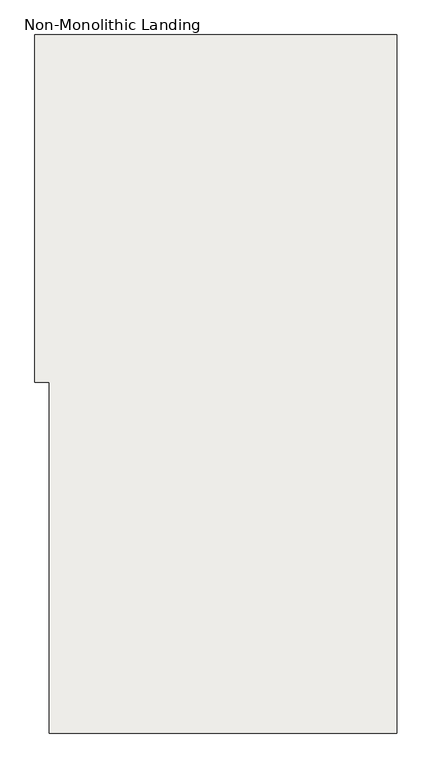
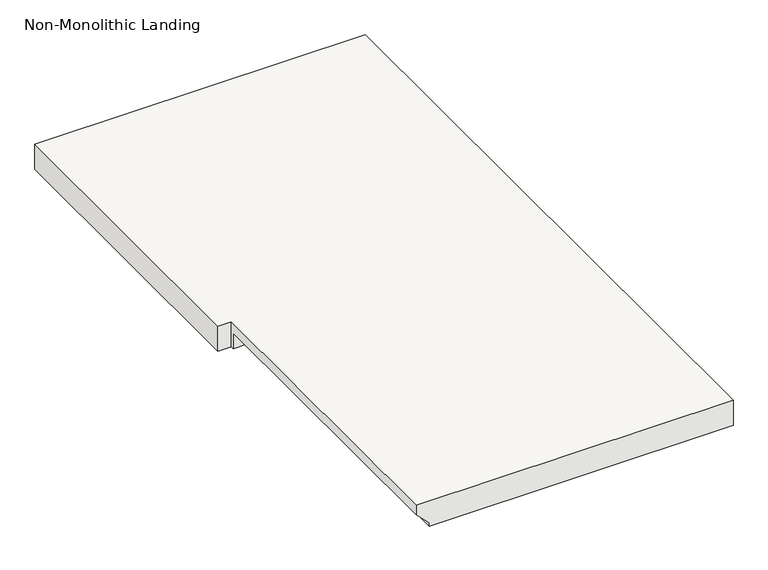
"""IFC4 building model written with IfcOpenShell, lengths in millimetres: slab geometry, Non-Monolithic Landing."""

from ifc_helpers import new_model, si_unit, origin, place, context, project, spatial, faceted_brep, source, transform, mapped, element, save


def non_monolithic_landing_067df1a0(model_context):
    return source(origin(), model_context, "Body", "Brep", [
        faceted_brep([(-2686.4237097, 3724.9480625, 4800.6), (-2686.4237097, 4950.7083475, 4800.6), (-3296.0237097, 4950.7083475, 4800.6), (-3321.4237097, 4950.7083475, 4800.6), (-3321.4237097, 4341.1083475, 4800.6), (-3296.0237097, 4341.1083475, 4800.6), (-3296.0237097, 3724.9480625, 4800.6), (-3270.6237097, 4334.5480625, 4749.8), (-3296.0237097, 4334.5480625, 4749.8), (-3296.0237097, 4341.1083475, 4749.8), (-3321.4237097, 4341.1083475, 4749.8), (-3321.4237097, 4950.7083475, 4749.8), (-3296.0237097, 4950.7083475, 4749.8), (-2686.4237097, 4950.7083475, 4749.8), (-2686.4237097, 3724.9480625, 4749.8), (-3270.6237097, 3724.9480625, 4749.8), (-3296.0237097, 4334.5480625, 4781.55), (-3296.0237097, 3724.9480625, 4781.55), (-3270.6237097, 3724.9480625, 4756.15), (-3270.6237097, 4334.5480625, 4756.15)], [[[0, 1, 2, 3, 4, 5, 6]], [[7, 8, 9, 10, 11, 12, 13, 14, 15]], [[2, 1, 13, 12]], [[4, 3, 11, 10]], [[3, 2, 12, 11]], [[6, 5, 9, 8, 16, 17]], [[0, 6, 17, 18, 15, 14]], [[18, 17, 16, 19]], [[8, 7, 19, 16]], [[7, 15, 18, 19]], [[1, 0, 14, 13]], [[5, 4, 10, 9]]]),
    ])


if __name__ == "__main__":
    model = new_model("IFC4")
    model_context = context("Model", 3, world=origin())
    ifc_project = project(units=[si_unit("LENGTHUNIT", "METRE", prefix="MILLI")], contexts=[model_context])
    site = spatial("IfcSite", under=ifc_project)
    building = spatial("IfcBuilding", under=site)
    placement = place(None, origin())
    non_monolithic_landing_shape = non_monolithic_landing_067df1a0(model_context)
    element("IfcSlab", 1, ObjectType="Non-Monolithic Landing", at=placement, inside=building, context=model_context, shape_type="MappedRepresentation", body=[
        mapped(non_monolithic_landing_shape, transform((0.0, 0.0, 0.0), x_axis=(1.0, 0.0, 0.0), y_axis=(0.0, 1.0, 0.0), z_axis=(0.0, 0.0, 1.0))),
    ])
    save(model, "model.ifc")
